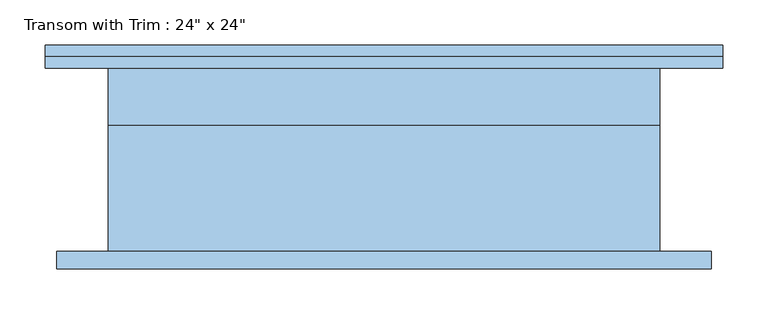
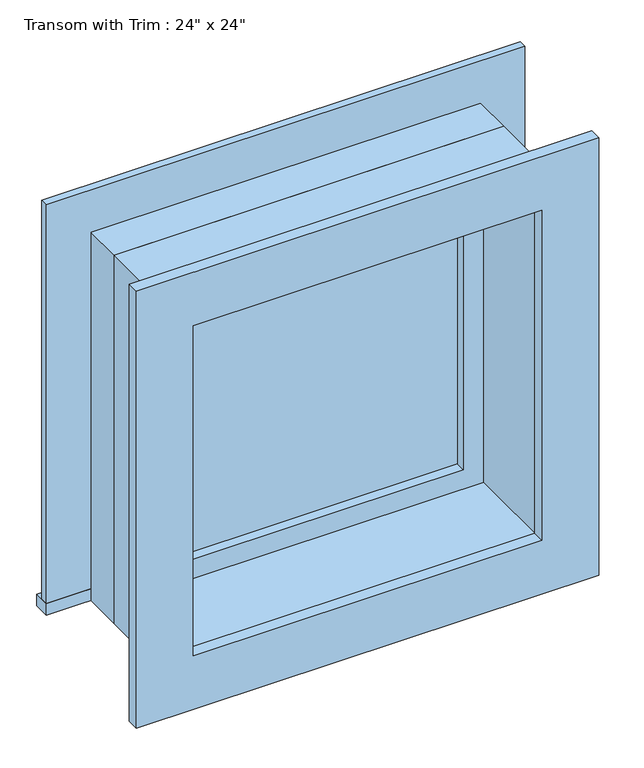
"""IFC4 building model written with IfcOpenShell, lengths in millimetres: window geometry."""

from ifc_helpers import new_model, si_unit, frame, origin, place, context, project, spatial, polyline, outline, extrude, source, transform, mapped, element, save


def window_e41d21a6(model_context):
    return source(origin(), model_context, "Body", "SweptSolid", [
        extrude(outline(polyline([(-412.75, 127.0), (336.55, 127.0), (336.55, 101.6), (-412.75, 101.6), (-412.75, 127.0)])), frame((0.0, 0.0, 2159.0), z_axis=(0.0, 0.0, 1.0), x_axis=(1.0, 0.0, 0.0)), (0.0, 0.0, 1.0), 19.05),
        extrude(outline(polyline([(2749.55, -323.85), (2749.55, 247.65), (2178.05, 247.65), (2178.05, 336.55), (2838.45, 336.55), (2838.45, -412.75), (2178.05, -412.75), (2178.05, -323.85), (2749.55, -323.85)])), frame((0.0, 101.6, 0.0), z_axis=(0.0, 1.0, 0.0), x_axis=(0.0, 0.0, 1.0)), (0.0, 0.0, 1.0), 12.7),
        extrude(outline(polyline([(2825.75, 323.85), (2825.75, -400.05), (2101.85, -400.05), (2101.85, 323.85), (2825.75, 323.85)]), holes=[polyline([(2736.85, 234.95), (2190.75, 234.95), (2190.75, -311.15), (2736.85, -311.15), (2736.85, 234.95)])]), frame((0.0, -120.65, 0.0), z_axis=(0.0, 1.0, 0.0), x_axis=(0.0, 0.0, 1.0)), (0.0, 0.0, 1.0), 19.05),
        extrude(outline(polyline([(203.2, 53.975), (-279.4, 53.975), (-279.4, 66.675), (203.2, 66.675), (203.2, 53.975)])), frame((0.0, 0.0, 2222.5), z_axis=(0.0, 0.0, 1.0), x_axis=(1.0, 0.0, 0.0)), (0.0, 0.0, 1.0), 482.6),
        extrude(outline(polyline([(2749.55, -323.85), (2178.05, -323.85), (2178.05, 247.65), (2749.55, 247.65), (2749.55, -323.85)]), holes=[polyline([(2705.1, -279.4), (2705.1, 203.2), (2222.5, 203.2), (2222.5, -279.4), (2705.1, -279.4)])]), frame((0.0, 38.1, 0.0), z_axis=(0.0, 1.0, 0.0), x_axis=(0.0, 0.0, 1.0)), (0.0, 0.0, 1.0), 44.45),
        extrude(outline(polyline([(2768.6, -342.9), (2159.0, -342.9), (2159.0, 266.7), (2768.6, 266.7), (2768.6, -342.9)]), holes=[polyline([(2736.85, -311.15), (2736.85, 234.95), (2190.75, 234.95), (2190.75, -311.15), (2736.85, -311.15)])]), frame((0.0, -101.6, 0.0), z_axis=(0.0, 1.0, 0.0), x_axis=(0.0, 0.0, 1.0)), (0.0, 0.0, 1.0), 139.7),
        extrude(outline(polyline([(2768.6, 266.7), (2768.6, -342.9), (2159.0, -342.9), (2159.0, 266.7), (2768.6, 266.7)]), holes=[polyline([(2749.55, 247.65), (2178.05, 247.65), (2178.05, -323.85), (2749.55, -323.85), (2749.55, 247.65)])]), frame((0.0, 38.1, 0.0), z_axis=(0.0, 1.0, 0.0), x_axis=(0.0, 0.0, 1.0)), (0.0, 0.0, 1.0), 63.5),
    ])


if __name__ == "__main__":
    model = new_model("IFC4")
    model_context = context("Model", 3, world=origin())
    ifc_project = project(units=[si_unit("LENGTHUNIT", "METRE", prefix="MILLI")], contexts=[model_context])
    site = spatial("IfcSite", under=ifc_project)
    building = spatial("IfcBuilding", under=site)
    placement = place(None, origin())
    window_shape = window_e41d21a6(model_context)
    element("IfcWindow", 1, ObjectType="Transom with Trim : 24\" x 24\"", at=placement, inside=building, context=model_context, shape_type="MappedRepresentation", body=[
        mapped(window_shape, transform((0.0, 0.0, 0.0), x_axis=(1.0, 0.0, 0.0), y_axis=(0.0, 1.0, 0.0), z_axis=(0.0, 0.0, 1.0))),
    ])
    save(model, "model.ifc")

# Revit data of these elements
# Type "Transom with Trim : 24\" x 24\""
#   Type Mark = "25"
#   Construction Type Id = "GSP4R"
#   Assembly Code = "B2020100"
#   Analytic Construction = "1/8 in Pilkington single glazing"
#   Visual Light Transmittance = 0.9
#   Solar Heat Gain Coefficient = 0.78
#   Heat Transfer Coefficient (U) = 0.6496 BTU/(h·ft²·°F)
#   Height = 2' - 0"
#   Default Sill Height = 7' - 1"
#   Trim Projection - Ext. = 0' - 0 1/2"
#   Trim Projection - Int. = 0' - 0 3/4"
#   Trim Width - Exterior = 0' - 3 1/2"
#   Trim Width - Interior = 0' - 3 1/2"
#   Width = 2' - 0"
#   Window Inset = 0' - 0 3/4"
#   Define Thermal Properties by = 1
#   Glass Pane Material = Glass
#   Sash Material = Sash
#   Trim Exterior Material = Trim
#   Trim Interior Material = Trim
#   Wall Closure = (empty or 0)
# Element 1 (IfcWindow, "Transom with Trim : 24\" x 24\"")
#   Materials on its faces: "Sash", "Trim", "Glass"
# Materials
#   "Glass": class "Glass", colour RGB 0 128 192, transparency 0.75, Description = "Soda Lime Glass", Cost = 0
#   "Sash": class "Wood", colour RGB 224 178 126, transparency 0
#   "Trim": class "Wood", colour RGB 224 178 126, transparency 0
